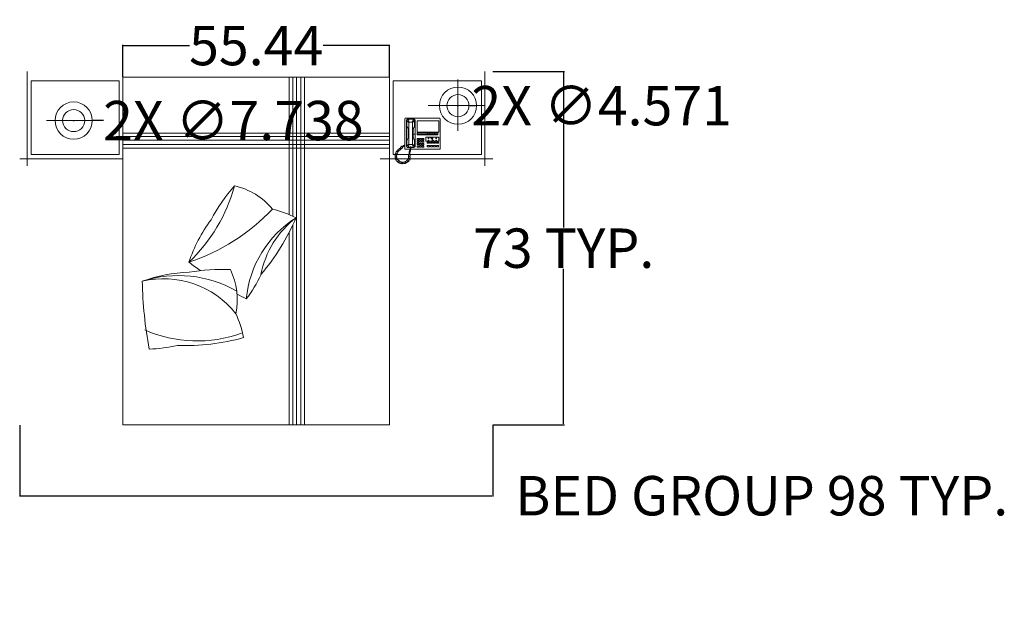
# Model space of a CAD drawing. Units: inches. Extents: x -254 to 1961, y 86 to 3025.
# Tile 1 of 6: x -254 to -50, y 432 to 557. Entities that reach past the tile are written whole.
import ezdxf

# ---------------------------------------------------------------- set-up
doc = ezdxf.new("R2010")
doc.units = ezdxf.units.IN
doc.header["$MEASUREMENT"] = 0
doc.layers.add('A-ANNO-DIMS', color=2, linetype='Continuous', lineweight=18)
doc.layers.add('FURNITURE', color=151, linetype='Continuous', lineweight=13)
doc.styles.get("Standard").update_dxf_attribs({"font": 'arial.ttf'})
doc.dimstyles.get("Standard").update_dxf_attribs({"dimtxt": 8.18, "dimasz": 0.18, "dimexe": 0.18, "dimexo": 0.0625, "dimgap": 0.09, "dimtad": 0, "dimtih": 1, "dimtoh": 1, "dimdec": 1, "dimzin": 0, "dimdsep": 46, "dimlunit": 3, "dimtxsty": 'Standard', "dimcen": 0.09, "dimadec": 0, "dimazin": 0, "dimtfac": 1, "dimtdec": 1, "dimtofl": 0, "dimtmove": 0, "dimatfit": 3, "dimfxl": 1, "dimtolj": 1, "dimtzin": 0, "dimarcsym": 0})

# ---------------------------------------------------------------- blocks, each defined once
blk = doc.blocks.new('BED-DOUBLE-NIGHTSTANDS')
for p, q in [((1.58, 73.32), (1.58, 53.78)), ((21.4, 73.32), (21.4, 53.78)), ((76.84, 72.19), (21.4, 72.19)), ((21.4, 72.19), (21.4, 0)), ((55.98, 43.63), (55.98, 72.19)), ((56.73, 43.3), (56.73, 72.19)), ((57.47, 0), (57.47, 72.19)), ((58.37, 0), (58.37, 72.19)), ((59.13, 0), (59.13, 72.19)), ((76.84, 73.32), (76.84, 53.78)), ((76.84, 0), (76.84, 72.19)), ((91.03, 61.02), (91.03, 71.64)), ((96.61, 73.32), (96.61, 53.78)), ((20.68, 71.37), (2.35, 71.37)), ((2.35, 71.37), (2.35, 56.1)), ((20.68, 56.1), (20.68, 71.37)), ((77.56, 56.1), (77.56, 71.37)), ((77.56, 71.37), (95.89, 71.37)), ((95.89, 71.37), (95.89, 56.1)), ((96.71, 66.24), (84.84, 66.24)), ((79.99, 63.51), (80.08, 63.61)), ((79.99, 57.27), (79.99, 63.51)), ((80.08, 63.61), (87.23, 63.61)), ((80.58, 63.47), (80.35, 63.24)), ((80.67, 63.42), (80.49, 63.33)), ((81.94, 63.47), (80.58, 63.47)), ((81.76, 63.42), (80.67, 63.42)), ((80.9, 62.84), (80.67, 63.42)), ((81.76, 63.42), (81.53, 62.84)), ((81.94, 63.33), (81.76, 63.42)), ((82.12, 63.24), (81.94, 63.47)), ((87.23, 63.61), (87.32, 63.51)), ((87.32, 63.51), (87.32, 57.27)), ((5.54, 63.15), (17.4, 63.15)), ((80.35, 63.24), (80.35, 57.81)), ((80.49, 63.33), (80.44, 63.15)), ((80.85, 62.75), (80.44, 63.15)), ((80.44, 63.15), (80.44, 61.93)), ((80.44, 61.93), (80.54, 61.7)), ((80.54, 61.7), (80.67, 61.48)), ((80.67, 61.48), (80.72, 61.16)), ((80.9, 62.84), (80.85, 62.75)), ((80.85, 62.75), (80.85, 60.71)), ((81.53, 62.84), (80.9, 62.84)), ((81.58, 62.75), (81.53, 62.84)), ((81.98, 63.15), (81.58, 62.75)), ((81.58, 62.75), (81.58, 60.71)), ((81.71, 61.16), (81.76, 61.48)), ((81.76, 61.48), (81.89, 61.7)), ((81.89, 61.7), (81.98, 61.93)), ((81.98, 63.15), (81.94, 63.33)), ((81.98, 61.93), (81.98, 63.15)), ((82.12, 57.77), (82.12, 63.24)), ((82.53, 60.71), (82.53, 63.11)), ((82.53, 63.11), (87.05, 63.11)), ((87.05, 63.11), (87.05, 60.71)), ((21.4, 60.55), (76.84, 60.55)), ((21.4, 59.81), (76.84, 59.81)), ((80.67, 59.53), (80.54, 59.31)), ((80.72, 59.85), (80.67, 59.53)), ((80.72, 61.16), (80.72, 60.71)), ((80.72, 60.71), (80.72, 59.85)), ((80.85, 60.71), (80.85, 58.26)), ((81.58, 60.71), (81.58, 58.26)), ((81.71, 60.71), (81.71, 61.16)), ((81.71, 59.85), (81.71, 60.71)), ((82.12, 60.34), (81.71, 60.34)), ((81.76, 59.53), (81.71, 59.85)), ((81.89, 59.31), (81.76, 59.53)), ((87.05, 60.71), (82.53, 60.71)), ((82.53, 60.17), (82.53, 60.62)), ((82.53, 60.62), (86.87, 60.62)), ((86.87, 60.34), (82.53, 60.34)), ((86.87, 60.17), (82.53, 60.17)), ((82.89, 59.44), (82.53, 59.44)), ((82.53, 59.44), (82.53, 59.17)), ((82.89, 59.17), (82.89, 59.44)), ((83.07, 59.44), (83.07, 59.17)), ((83.43, 59.44), (83.07, 59.44)), ((83.43, 59.17), (83.43, 59.44)), ((83.97, 59.44), (83.61, 59.44)), ((83.61, 59.44), (83.61, 59.17)), ((83.97, 59.17), (83.97, 59.44)), ((84.38, 58.85), (84.38, 59.67)), ((84.38, 59.67), (87.05, 59.67)), ((84.73, 60.17), (84.56, 60.34)), ((84.7, 60.62), (84.7, 60.17)), ((84.83, 59.44), (84.83, 59.58)), ((84.83, 59.58), (84.97, 59.58)), ((84.97, 59.44), (84.83, 59.44)), ((84.97, 59.58), (84.97, 59.44)), ((85.06, 60.62), (85.06, 60.17)), ((86.04, 58.85), (85.23, 59.67)), ((85.42, 60.62), (85.42, 60.17)), ((85.65, 59.44), (85.65, 59.58)), ((85.65, 59.58), (85.79, 59.58)), ((85.79, 59.44), (85.65, 59.44)), ((85.79, 60.62), (85.79, 60.17)), ((85.79, 59.58), (85.79, 59.44)), ((86.15, 60.62), (86.15, 60.17)), ((86.46, 59.44), (86.46, 59.58)), ((86.46, 59.58), (86.6, 59.58)), ((86.6, 59.44), (86.46, 59.44)), ((86.51, 60.62), (86.51, 60.17)), ((86.6, 59.58), (86.6, 59.44)), ((86.87, 60.62), (86.87, 60.17)), ((87.05, 59.67), (87.05, 58.85)), ((21.4, 59.06), (76.84, 59.06)), ((21.4, 58.17), (76.84, 58.17)), ((21.4, 57.41), (76.84, 57.41)), ((78.72, 57.24), (78.93, 57.44)), ((78.93, 57.44), (79.18, 57.31)), ((79.08, 57.58), (79.2, 57.7)), ((79.18, 57.31), (79.08, 57.58)), ((79.56, 57.55), (79.19, 57.22)), ((79.2, 57.7), (79.31, 57.62)), ((79.25, 57.75), (79.33, 57.83)), ((79.31, 57.62), (79.25, 57.75)), ((79.33, 57.83), (79.5, 57.77)), ((79.56, 57.64), (79.47, 57.65)), ((79.47, 57.65), (79.56, 57.55)), ((79.5, 57.77), (79.59, 57.85)), ((79.61, 57.7), (79.56, 57.64)), ((79.59, 57.85), (79.72, 57.98)), ((79.79, 57.85), (79.61, 57.7)), ((79.72, 57.98), (79.99, 58.08)), ((79.99, 57.9), (79.79, 57.85)), ((80.08, 57.18), (79.99, 57.27)), ((80.35, 57.81), (80.58, 57.54)), ((80.54, 59.31), (80.44, 59.08)), ((80.44, 59.08), (80.44, 57.86)), ((80.44, 57.86), (80.85, 58.26)), ((80.49, 57.68), (80.44, 57.86)), ((80.67, 57.59), (80.49, 57.68)), ((80.58, 57.54), (81.11, 57.54)), ((80.67, 57.59), (80.9, 58.17)), ((81.11, 57.59), (80.67, 57.59)), ((80.85, 58.26), (80.9, 58.17)), ((80.9, 58.17), (81.53, 58.17)), ((81.03, 57.07), (81.1, 57.36)), ((81.1, 57.36), (81.12, 57.72)), ((81.12, 57.72), (81.26, 57.72)), ((81.25, 57.33), (81.14, 56.87)), ((81.26, 57.72), (81.25, 57.33)), ((81.76, 57.59), (81.26, 57.59)), ((81.26, 57.54), (81.89, 57.54)), ((81.58, 58.26), (81.53, 58.17)), ((81.53, 58.17), (81.76, 57.59)), ((81.98, 57.86), (81.58, 58.26)), ((81.76, 57.59), (81.94, 57.68)), ((81.98, 59.08), (81.89, 59.31)), ((81.89, 57.54), (82.12, 57.77)), ((81.94, 57.68), (81.98, 57.86)), ((81.98, 57.86), (81.98, 59.08)), ((82.53, 59.17), (82.89, 59.17)), ((82.89, 58.94), (82.53, 58.94)), ((82.53, 58.94), (82.53, 58.67)), ((82.53, 58.67), (82.89, 58.67)), ((82.53, 58.45), (82.53, 58.17)), ((82.89, 58.45), (82.53, 58.45)), ((82.53, 58.17), (82.89, 58.17)), ((82.53, 57.9), (82.53, 57.63)), ((82.89, 57.9), (82.53, 57.9)), ((82.53, 57.63), (82.89, 57.63)), ((82.89, 58.67), (82.89, 58.94)), ((82.89, 58.17), (82.89, 58.45)), ((82.89, 57.63), (82.89, 57.9)), ((83.07, 59.17), (83.43, 59.17)), ((83.43, 58.94), (83.07, 58.94)), ((83.07, 58.94), (83.07, 58.67)), ((83.07, 58.67), (83.43, 58.67)), ((83.07, 58.4), (83.07, 58.13)), ((83.43, 58.4), (83.07, 58.4)), ((83.07, 58.13), (83.43, 58.13)), ((83.43, 57.9), (83.07, 57.9)), ((83.07, 57.9), (83.07, 57.63)), ((83.07, 57.63), (83.43, 57.63)), ((83.43, 58.67), (83.43, 58.94)), ((83.43, 58.13), (83.43, 58.4)), ((83.43, 57.63), (83.43, 57.9)), ((83.61, 59.17), (83.97, 59.17)), ((83.97, 58.94), (83.61, 58.94)), ((83.61, 58.94), (83.61, 58.67)), ((83.61, 58.67), (83.97, 58.67)), ((83.97, 58.4), (83.61, 58.4)), ((83.61, 58.4), (83.61, 58.13)), ((83.61, 58.13), (83.97, 58.13)), ((83.97, 57.9), (83.61, 57.9)), ((83.61, 57.9), (83.61, 57.63)), ((83.61, 57.63), (83.97, 57.63)), ((83.97, 58.67), (83.97, 58.94)), ((83.97, 58.13), (83.97, 58.4)), ((83.97, 57.63), (83.97, 57.9)), ((87.05, 58.85), (84.38, 58.85)), ((84.65, 58.45), (84.65, 58.63)), ((84.65, 58.63), (85.11, 58.63)), ((85.11, 58.45), (84.65, 58.45)), ((85.11, 57.95), (84.65, 57.95)), ((84.65, 57.95), (84.65, 57.68)), ((84.65, 57.68), (85.11, 57.68)), ((84.83, 58.94), (84.83, 59.08)), ((84.83, 59.08), (84.97, 59.08)), ((84.97, 58.94), (84.83, 58.94)), ((84.97, 59.08), (84.97, 58.94)), ((85.11, 58.63), (85.11, 58.45)), ((85.11, 57.68), (85.11, 57.95)), ((85.29, 58.63), (85.74, 58.63)), ((85.29, 58.45), (85.29, 58.63)), ((85.74, 58.45), (85.29, 58.45)), ((85.29, 57.95), (85.29, 57.68)), ((85.74, 57.95), (85.29, 57.95)), ((85.29, 57.68), (85.74, 57.68)), ((85.65, 58.94), (85.65, 59.08)), ((85.65, 59.08), (85.79, 59.08)), ((85.79, 58.94), (85.65, 58.94)), ((85.74, 58.63), (85.74, 58.45)), ((85.74, 57.68), (85.74, 57.95)), ((85.79, 59.08), (85.79, 58.94)), ((85.92, 58.63), (86.37, 58.63)), ((85.92, 58.45), (85.92, 58.63)), ((86.37, 58.45), (85.92, 58.45)), ((85.92, 57.95), (85.92, 57.68)), ((86.37, 57.95), (85.92, 57.95)), ((85.92, 57.68), (86.37, 57.68)), ((86.37, 58.52), (86.27, 58.63)), ((86.37, 58.63), (86.37, 58.45)), ((86.37, 57.68), (86.37, 57.95)), ((86.46, 58.94), (86.46, 59.08)), ((86.46, 59.08), (86.6, 59.08)), ((86.6, 58.94), (86.46, 58.94)), ((86.55, 58.63), (87.01, 58.63)), ((86.55, 58.45), (86.55, 58.63)), ((87.01, 58.45), (86.55, 58.45)), ((86.55, 57.95), (86.55, 57.68)), ((87.01, 57.95), (86.55, 57.95)), ((86.55, 57.68), (87.01, 57.68)), ((86.6, 59.08), (86.6, 58.94)), ((87.01, 57.89), (86.95, 57.95)), ((87.01, 58.63), (87.01, 58.45)), ((87.01, 57.68), (87.01, 57.95)), ((87.32, 57.27), (87.23, 57.18)), ((2.35, 56.1), (20.68, 56.1)), ((95.89, 56.1), (77.56, 56.1)), ((77.91, 55.74), (77.96, 55.97)), ((78.19, 55.65), (77.91, 55.74)), ((77.96, 55.97), (78.2, 55.97)), ((77.96, 55.52), (78.19, 55.65)), ((77.99, 55.33), (77.96, 55.52)), ((78.28, 55.34), (77.99, 55.33)), ((78.01, 56.15), (78.07, 56.36)), ((78.2, 55.97), (78.01, 56.15)), ((78.06, 55.09), (78.28, 55.34)), ((78.07, 56.36), (78.37, 56.35)), ((78.1, 56.45), (78.18, 56.73)), ((78.37, 56.35), (78.1, 56.45)), ((78.18, 56.73), (78.46, 56.7)), ((78.38, 55.31), (78.24, 55.31)), ((78.59, 56.7), (78.29, 55.84)), ((78.29, 55.84), (78.41, 55.15)), ((78.39, 56.9), (78.56, 57.08)), ((78.46, 56.7), (78.39, 56.9)), ((78.56, 57.08), (78.77, 56.95)), ((79.19, 57.22), (78.6, 56.71)), ((78.77, 56.95), (78.72, 57.24)), ((81.06, 57.18), (80.08, 57.18)), ((80.38, 54.83), (80.73, 55.27)), ((80.73, 55.27), (80.78, 55.85)), ((80.74, 56.06), (80.9, 56.18)), ((80.78, 55.85), (80.74, 56.06)), ((81.11, 55.38), (80.81, 55.35)), ((80.81, 55.35), (81.07, 55.15)), ((81.13, 55.83), (80.87, 55.78)), ((80.87, 55.78), (81.12, 55.63)), ((80.9, 56.41), (80.92, 56.63)), ((80.9, 56.18), (80.9, 56.41)), ((80.92, 56.63), (81.03, 57.07)), ((81.04, 56.2), (81.01, 56.15)), ((81.01, 56.15), (81.12, 56.05)), ((81.14, 56.87), (81.03, 56.44)), ((81.03, 56.44), (81.04, 56.2)), ((81.12, 55.63), (81.11, 55.38)), ((81.12, 56.05), (81.13, 55.83)), ((87.23, 57.18), (81.22, 57.18)), ((0, 55.17), (21.4, 55.17)), ((98.24, 55.17), (74.88, 55.17)), ((78.13, 54.91), (78.06, 55.09)), ((78.4, 54.99), (78.13, 54.91)), ((78.27, 54.75), (78.4, 54.99)), ((78.39, 54.64), (78.27, 54.75)), ((78.64, 54.75), (78.39, 54.64)), ((78.41, 55.15), (78.82, 54.76)), ((78.53, 54.5), (78.64, 54.75)), ((78.68, 54.37), (78.53, 54.5)), ((78.87, 54.61), (78.68, 54.37)), ((78.82, 54.76), (79.35, 54.53)), ((78.84, 54.33), (78.87, 54.61)), ((78.99, 54.26), (78.84, 54.33)), ((79.2, 54.44), (78.99, 54.26)), ((79.21, 54.2), (79.2, 54.44)), ((79.38, 54.15), (79.21, 54.2)), ((79.35, 54.53), (79.9, 54.57)), ((79.49, 54.44), (79.38, 54.15)), ((79.55, 54.18), (79.49, 54.44)), ((79.71, 54.2), (79.55, 54.18)), ((79.82, 54.44), (79.71, 54.2)), ((79.93, 54.2), (79.82, 54.44)), ((79.9, 54.57), (80.38, 54.83)), ((80.13, 54.25), (79.93, 54.2)), ((80.32, 54.37), (80.1, 54.55)), ((80.1, 54.55), (80.13, 54.25)), ((80.49, 54.48), (80.32, 54.37)), ((80.67, 54.57), (80.46, 54.73)), ((80.46, 54.73), (80.49, 54.48)), ((80.8, 54.74), (80.67, 54.57)), ((80.95, 54.94), (80.68, 54.99)), ((80.68, 54.99), (80.8, 54.74)), ((81.07, 55.15), (80.95, 54.94)), ((56.73, 0), (56.73, 41.48)), ((55.98, 0), (55.98, 39.96)), ((21.4, 0), (76.84, 0))]:
    blk.add_line(p, q)
for centre, radius in [((91.03, 66.24), 3.87), ((91.03, 66.24), 2.29), ((11.21, 63.15), 3.87), ((11.21, 63.15), 2.29)]:
    blk.add_circle(centre, radius)
for centre, radius, start, end in [((11.42, 58.69), 34.44, 313.5807, 344.664), ((74.12, 23.89), 39.12, 138.9434, 151.5029), ((41.57, 35.76), 14.16, 39.5375, 77.5218), ((21.54, 74.27), 42.76, 288.5712, 316.3694), ((69.36, 24.04), 22.39, 122.3105, 174.6609), ((14.94, 61.05), 46.14, 319.6791, 336.9358), ((69.1, 27.6), 19.32, 127.3136, 169.3014), ((47.53, 23.64), 21.7, 62.9638, 76.7966), ((64.75, 23.92), 31.18, 143.3149, 161.6473), ((87.82, 103.02), 87.02, 232.7582, 234.7034), ((36.16, 0.49), 31.18, 91.7513, 110.0837), ((32.98, 6.89), 24.09, 59.8649, 108.19), ((41.96, -6.88), 39.12, 87.3798, 99.9393), ((31.02, 26.01), 14.16, 347.9738, 25.9582), ((23.83, 43.59), 29.07, 323.0649, 334.741), ((29.97, 11.42), 18.9, 37.9983, 103.8151), ((112.46, 31.59), 87.02, 181.1946, 190.5116), ((87.82, 103.02), 87.02, 240.6207, 242.0752), ((25.24, 13.81), 21.7, 11.4002, 25.233), ((36.91, 44.65), 27.26, 246.3586, 289.7064), ((26.13, 44.77), 29.07, 271.5012, 283.1774), ((34.28, 62.58), 46.14, 268.1155, 285.3722)]:
    blk.add_arc(centre, radius, start, end)
blk = doc.blocks.new('*D20')
at = {"layer": 'A-ANNO-DIMS', "color": 0, "lineweight": -2, "transparency": 16777216}
for p, q in [((-254.31, 472.6), (-254.31, 457.75)), ((-156.07, 472.6), (-156.07, 457.75)), ((-254.13, 457.93), (-156.25, 457.93)), ((-156.07, 457.93), (-155.89, 457.93))]:
    blk.add_line(p, q, dxfattribs=at)
at = {"layer": 'A-ANNO-DIMS', "color": 0, "transparency": 16777216}
for points in [[(-254.13, 457.96), (-254.13, 457.9), (-254.31, 457.93)], [(-156.25, 457.96), (-156.25, 457.9), (-156.07, 457.93)]]:
    blk.add_solid(points, dxfattribs=at)
at = {"layer": 'Defpoints', "color": 0, "transparency": 16777216}
for p in [(-254.31, 472.66), (-156.07, 472.66), (-156.07, 457.93)]:
    blk.add_point(p, dxfattribs=at)
at = {"layer": 'A-ANNO-DIMS', "color": 0, "transparency": 16777216, "insert": (-100.2, 457.93), "char_height": 8.18, "attachment_point": 5}
blk.add_mtext('\\A1;BED GROUP 98 TYP.', dxfattribs=at)
blk = doc.blocks.new('*D21')
at = {"layer": 'A-ANNO-DIMS', "color": 0, "lineweight": -2, "transparency": 16777216}
for p, q in [((-156.01, 545.98), (-141.15, 545.98)), ((-141.33, 545.8), (-141.33, 513.59)), ((-141.33, 472.84), (-141.33, 505.05)), ((-156.01, 472.66), (-141.15, 472.66))]:
    blk.add_line(p, q, dxfattribs=at)
at = {"layer": 'A-ANNO-DIMS', "color": 0, "transparency": 16777216}
for points in [[(-141.36, 545.8), (-141.3, 545.8), (-141.33, 545.98)], [(-141.36, 472.84), (-141.3, 472.84), (-141.33, 472.66)]]:
    blk.add_solid(points, dxfattribs=at)
at = {"layer": 'Defpoints', "color": 0, "transparency": 16777216}
for p in [(-156.07, 545.98), (-141.33, 545.98), (-156.07, 472.66)]:
    blk.add_point(p, dxfattribs=at)
at = {"layer": 'A-ANNO-DIMS', "color": 0, "transparency": 16777216, "insert": (-141.33, 509.32), "char_height": 8.18, "attachment_point": 5}
blk.add_mtext('\\A1;73 TYP.', dxfattribs=at)
blk = doc.blocks.new('*D70')
at = {"layer": 'A-ANNO-DIMS', "color": 0, "lineweight": -2, "transparency": 16777216}
for p, q in [((-232.91, 544.92), (-232.91, 551.56)), ((-232.73, 551.38), (-219.06, 551.38)), ((-177.65, 551.38), (-191.31, 551.38)), ((-177.47, 544.92), (-177.47, 551.56))]:
    blk.add_line(p, q, dxfattribs=at)
at = {"layer": 'A-ANNO-DIMS', "color": 0, "transparency": 16777216}
for points in [[(-232.73, 551.41), (-232.73, 551.35), (-232.91, 551.38)], [(-177.65, 551.41), (-177.65, 551.35), (-177.47, 551.38)]]:
    blk.add_solid(points, dxfattribs=at)
at = {"layer": 'Defpoints', "color": 0, "transparency": 16777216}
for p in [(-177.47, 551.38), (-232.91, 544.86), (-177.47, 544.86)]:
    blk.add_point(p, dxfattribs=at)
at = {"layer": 'A-ANNO-DIMS', "color": 0, "transparency": 16777216, "insert": (-205.19, 551.38), "char_height": 8.18, "attachment_point": 5}
blk.add_mtext('\\A1;55.44', dxfattribs=at)
blk = doc.blocks.new('*D113')
at = {"layer": 'A-ANNO-DIMS', "color": 0, "lineweight": -2, "transparency": 16777216}
for p, q in [((-243.19, 535.81), (-243.01, 535.81)), ((-243.1, 535.72), (-243.1, 535.9)), ((-236.91, 535.81), (-239.05, 535.81))]:
    blk.add_line(p, q, dxfattribs=at)
at = {"layer": 'A-ANNO-DIMS', "color": 0, "transparency": 16777216}
blk.add_solid([(-239.05, 535.84), (-239.05, 535.78), (-239.23, 535.81)], dxfattribs=at)
at = {"layer": 'Defpoints', "color": 0, "transparency": 16777216}
for p in [(-246.97, 535.81), (-239.23, 535.81)]:
    blk.add_point(p, dxfattribs=at)
at = {"layer": 'A-ANNO-DIMS', "color": 0, "transparency": 16777216, "insert": (-209.92, 535.81), "char_height": 8.18, "attachment_point": 5}
blk.add_mtext('\\A1;2X ∅7.738', dxfattribs=at)
blk = doc.blocks.new('*D114')
at = {"layer": 'A-ANNO-DIMS', "color": 0, "lineweight": -2, "transparency": 16777216}
for p, q in [((-163.37, 538.91), (-163.19, 538.91)), ((-163.28, 538.82), (-163.28, 539)), ((-159.62, 538.9), (-160.81, 538.9))]:
    blk.add_line(p, q, dxfattribs=at)
at = {"layer": 'A-ANNO-DIMS', "color": 0, "transparency": 16777216}
blk.add_solid([(-160.81, 538.93), (-160.81, 538.87), (-160.99, 538.9)], dxfattribs=at)
at = {"layer": 'Defpoints', "color": 0, "transparency": 16777216}
for p in [(-165.56, 538.91), (-160.99, 538.9)]:
    blk.add_point(p, dxfattribs=at)
at = {"layer": 'A-ANNO-DIMS', "color": 0, "transparency": 16777216, "insert": (-133.43, 538.9), "char_height": 8.18, "attachment_point": 5}
blk.add_mtext('\\A1;2X ∅4.571', dxfattribs=at)

msp = doc.modelspace()

# ---------------------------------------------------------------- block references
at = {"layer": 'FURNITURE'}
msp.add_blockref('BED-DOUBLE-NIGHTSTANDS', (-254.3094, 472.6629), dxfattribs=at)

# ---------------------------------------------------------------- texts
at = {"layer": 'FURNITURE', "flags": 9}
for tag, p, s in [('YSIZE', (-214.004, 501.3773), '806.5825'), ('XSIZE', (-214.004, 501.3772), '855.2549'), ('ZSIZE', (-214.004, 501.3464), '0.0000')]:
    msp.add_attdef(tag, p, s, height=0.0198, rotation=270, dxfattribs=at)

# ---------------------------------------------------------------- dimensions: what is measured, and where the dimension line sits
at = {"layer": 'A-ANNO-DIMS'}
dim = msp.add_linear_dim(base=(-177.47196, 551.38033), p1=(-232.90698, 544.85552), p2=(-177.47196, 544.85552), dimstyle='Standard', override={"dimdec": 2, "dimlfac": 1, "dimrnd": 0, "dimzin": 0, "dimdsep": 46, "dimlunit": 2}, dxfattribs=at)
dim.commit()
dim.dimension.update_dxf_attribs({"geometry": '*D70', "text_midpoint": (-205.18947, 551.38033)})
for p1, p2, picture, middle in [((-165.5614, 538.906), (-160.9906, 538.905), '*D114', (-159.6194, 538.9047)), ((-246.96819, 535.80942), (-239.22972, 535.809), '*D113', (-236.90818, 535.80887))]:
    dim = msp.add_diameter_dim_2p(p1=p1, p2=p2, text='2X <>', dimstyle='Standard', override={"dimdec": 3, "dimlfac": 1, "dimrnd": 0, "dimzin": 0, "dimdsep": 46, "dimlunit": 2}, dxfattribs=at)
    dim.commit()
    dim.dimension.update_dxf_attribs({"geometry": picture, "text_midpoint": middle, "dimtype": 163})
dim = msp.add_linear_dim(base=(-141.3342, 545.9803), p1=(-156.07, 472.6626), p2=(-156.07, 545.9803), angle=90, text='<> TYP.', dimstyle='Standard', override={"dimdec": 0, "dimlfac": 1, "dimrnd": 0, "dimzin": 0, "dimdsep": 46, "dimlunit": 2}, dxfattribs=at)
dim.commit()
dim.dimension.update_dxf_attribs({"geometry": '*D21', "text_midpoint": (-141.3342, 509.3215)})
dim = msp.add_linear_dim(base=(-156.07, 457.9268), p1=(-254.3089, 472.6626), p2=(-156.07, 472.6626), text='BED GROUP <> TYP.', dimstyle='Standard', override={"dimdec": 0, "dimlfac": 1, "dimrnd": 0, "dimzin": 0, "dimdsep": 46, "dimlunit": 2}, dxfattribs=at)
dim.commit()
dim.dimension.update_dxf_attribs({"geometry": '*D20', "text_midpoint": (-100.1972, 457.9268)})

doc.saveas('drawing.dxf')
